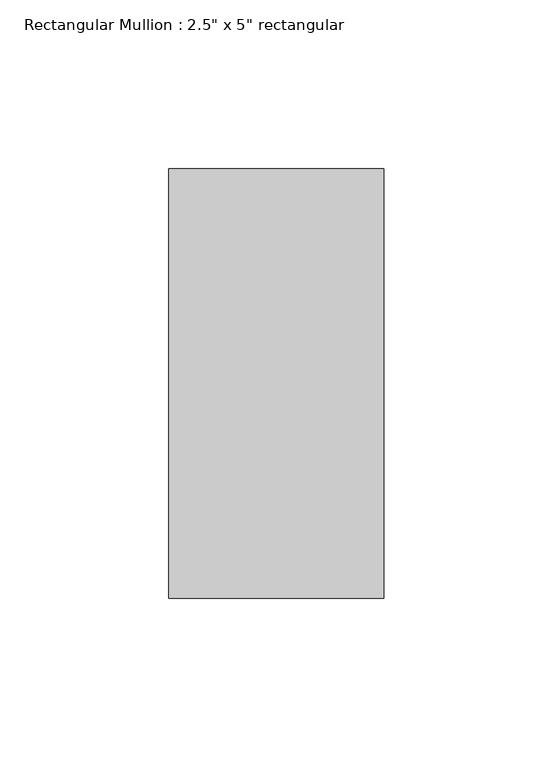
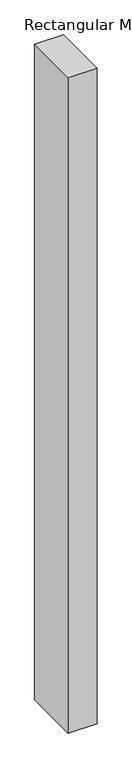
"""IFC4 building model written with IfcOpenShell, lengths in millimetres: member geometry."""

from ifc_helpers import new_model, si_unit, frame, origin, place, context, project, spatial, polyline, outline, extrude, source, transform, mapped, element, save


def member_0c289f97(model_context):
    return source(origin(), model_context, "Body", "SweptSolid", [
        extrude(outline(polyline([(0.0, 63.5), (0.0, -63.5), (-63.5, -63.5), (-63.5, 63.5), (0.0, 63.5)])), frame((0.0, 0.0, -1522.1131867), z_axis=(0.0, 0.0, 1.0), x_axis=(1.0, 0.0, 0.0)), (0.0, 0.0, 1.0), 1522.1131867),
    ])


if __name__ == "__main__":
    model = new_model("IFC4")
    model_context = context("Model", 3, world=origin())
    ifc_project = project(units=[si_unit("LENGTHUNIT", "METRE", prefix="MILLI")], contexts=[model_context])
    site = spatial("IfcSite", under=ifc_project)
    building = spatial("IfcBuilding", under=site)
    placement = place(None, origin())
    member_shape = member_0c289f97(model_context)
    element("IfcMember", 1, ObjectType="Rectangular Mullion : 2.5\" x 5\" rectangular", at=placement, inside=building, context=model_context, shape_type="MappedRepresentation", body=[
        mapped(member_shape, transform((0.0, 0.0, 0.0), x_axis=(1.0, 0.0, 0.0), y_axis=(0.0, 1.0, 0.0), z_axis=(0.0, 0.0, 1.0))),
    ])
    save(model, "model.ifc")

# Revit data of these elements
# Type "Rectangular Mullion : 2.5\" x 5\" rectangular"
#   built-in parameter 1007304 = 0.416667 (stored number, unit not read)
#   built-in parameter 1007301 = 0.104167 (stored number, unit not read)
#   built-in parameter 1007300 = 0.104167 (stored number, unit not read)
# Element 1 (IfcMember, "Rectangular Mullion : 2.5\" x 5\" rectangular")
#   Materials on its faces: "Aluminum"
# Materials
#   "Aluminum": class "Metal", colour RGB 247 247 247, transparency 0, Description = "Aluminum 6061", Cost = 0
